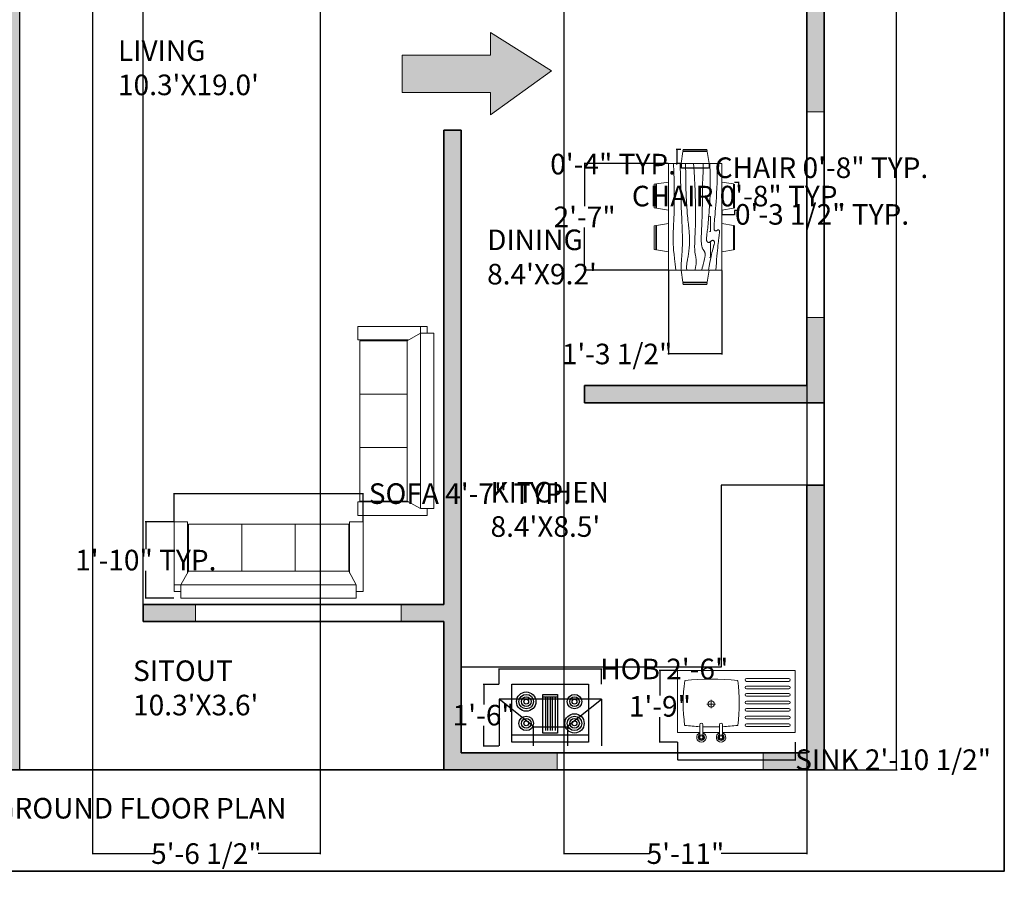
# Model space of a CAD drawing. Units: inches. Extents: x 717 to 1167, y 2046 to 2594.
# Tile 3 of 6: x 880 to 1167, y 2046 to 2298. Entities that reach past the tile are written whole.
import ezdxf

# ---------------------------------------------------------------- set-up
doc = ezdxf.new("R2010")
doc.units = ezdxf.units.IN
doc.header["$MEASUREMENT"] = 0
for name, color, linetype, lineweight in [('A-ANNO-DIMS', 2, 'Continuous', 18), ('A-ANNO-SYMB', 7, 'Continuous', 18), ('A-ANNO-TEXT', 7, 'Continuous', 25), ('A-ANNO-TTLB', 7, 'Continuous', 35), ('A-AREA-IDEN', 7, 'Continuous', 18), ('A-EQPM', 8, 'Continuous', 25), ('A-FLOR-CASE', 8, 'Continuous', 25), ('A-FLOR-FIXT', 8, 'Continuous', 18), ('A-FURN', 8, 'Continuous', 18), ('A-GLAZ', 4, 'Continuous', 18), ('A-WALL', 7, 'Continuous', 35), ('A-WALL-PATT', 140, 'Continuous', 13)]:
    doc.layers.add(name, color=color, linetype=linetype, lineweight=lineweight)
doc.styles.get("Standard").update_dxf_attribs({"font": 'arial.ttf'})
doc.dimstyles.get("Standard").update_dxf_attribs({"dimtxt": 6, "dimasz": 0.18, "dimexe": 0.18, "dimexo": 0.0625, "dimgap": 0.09, "dimtad": 0, "dimtih": 1, "dimtoh": 1, "dimdec": 1, "dimzin": 0, "dimdsep": 46, "dimlunit": 3, "dimtxsty": 'Standard', "dimcen": 0.09, "dimadec": 0, "dimazin": 0, "dimtfac": 1, "dimtdec": 1, "dimtofl": 0, "dimtmove": 0, "dimatfit": 3, "dimfxl": 1, "dimtolj": 1, "dimtzin": 0, "dimarcsym": 0})

# ---------------------------------------------------------------- blocks, each defined once
blk = doc.blocks.new('chimmne')
for p, q in [((17.89, 6.07), (-18.11, 6.07)), ((-18.11, 6.07), (-18.11, -10.43)), ((-6.16, -3.43), (-18.11, 6.07)), ((5.94, -3.43), (17.89, 6.07)), ((17.89, 6.07), (17.89, -10.43)), ((-6.16, -3.43), (-6.16, -10.43)), ((5.94, -3.43), (5.94, -10.43)), ((5.94, -3.82), (-6.16, -3.82))]:
    blk.add_line(p, q)
for points in [[(-13.61, -9.12), (-13.61, 11.28), (13.39, 11.28), (13.39, -9.12)], [(-2.66, -5.87), (-2.66, 7.73), (2.44, 7.73), (2.44, -5.87)]]:
    blk.add_lwpolyline(points, close=True)
for points in [[(-2.66, 6.88), (2.44, 6.88)], [(-1.81, 6.88), (-1.81, -5.02)], [(-0.96, -5.02), (-0.96, 6.88)], [(-0.11, 6.88), (-0.11, -5.02)], [(0.74, -5.02), (0.74, 6.88)], [(1.59, 6.88), (1.59, -5.02)], [(13.39, -6.57), (-13.61, -6.57)]]:
    blk.add_lwpolyline(points)
for centre, radius in [((-8.55, 5.18), 3.4), ((-8.55, 5.18), 2.55), ((8.44, 5.18), 2.55), ((-8.55, 5.18), 1.7), ((-8.55, 5.18), 0.85), ((8.44, 5.18), 1.7), ((8.44, 5.18), 0.85), ((-8.55, -2.47), 2.55), ((8.44, -2.47), 3.4), ((8.44, -2.47), 2.55), ((-8.55, -2.47), 1.7), ((-8.55, -2.47), 0.85), ((8.44, -2.47), 1.7), ((8.44, -2.47), 0.85)]:
    blk.add_circle(centre, radius)
blk = doc.blocks.new('A$C799204C7')
for p, q in [((0, 34.2), (17.99, 34.2)), ((0, 0), (0, 34.2)), ((2.32, 20.01), (2.32, 32.27)), ((3.13, 20.01), (3.13, 32.27)), ((4.48, 20.01), (4.48, 32.27)), ((5.29, 20.01), (5.29, 32.27)), ((6.64, 20.01), (6.64, 32.27)), ((7.45, 20.01), (7.45, 32.27)), ((8.85, 20.01), (8.85, 32.27)), ((9.66, 20.01), (9.66, 32.27)), ((11.01, 20.01), (11.01, 32.27)), ((11.82, 20.01), (11.82, 32.27)), ((13.22, 20.01), (13.22, 32.27)), ((14.03, 20.01), (14.03, 32.27)), ((15.42, 20.01), (15.42, 32.27)), ((16.24, 20.01), (16.24, 32.27)), ((17.99, 13.08), (17.99, 34.2)), ((18.59, 13.08), (15.71, 13.08)), ((15.71, 12.17), (18.59, 12.17)), ((17.99, 7.36), (17.99, 12.17)), ((8.52, 9.77), (10.9, 9.77)), ((9.73, 11), (9.73, 8.54)), ((18.59, 7.36), (15.71, 7.36)), ((15.71, 6.45), (18.59, 6.45)), ((17.99, 0), (17.99, 6.45)), ((0, 0), (17.99, 0))]:
    blk.add_line(p, q)
for centre, radius in [((19.38, 12.62), 0.684), ((19.38, 12.62), 0.456), ((9.7, 9.77), 0.916), ((19.38, 6.91), 0.684), ((19.38, 6.91), 0.456)]:
    blk.add_circle(centre, radius)
for centre, radius, start, end in [((2.72, 32.27), 0.407, 0, 180), ((4.88, 32.27), 0.407, 0, 180), ((7.05, 32.27), 0.407, 0, 180), ((9.25, 32.27), 0.407, 0, 180), ((11.42, 32.27), 0.407, 0, 180), ((13.62, 32.27), 0.407, 0, 180), ((15.83, 32.27), 0.407, 0, 180), ((2.72, 20.01), 0.407, 180, 0), ((67.33, 9.77), 64.88, 173.1952, 186.8048), ((9.53, -30.19), 48.1, 82.3437, 97.8966), ((4.88, 20.01), 0.407, 180, 0), ((7.05, 20.01), 0.407, 180, 0), ((9.25, 20.01), 0.407, 180, 0), ((11.42, 20.01), 0.407, 180, 0), ((13.62, 20.01), 0.407, 180, 0), ((15.83, 20.01), 0.407, 180, 0), ((-48.51, 9.77), 64.88, 2.9208, 6.8048), ((15.71, 12.62), 0.456, 90, 270), ((-48.51, 9.77), 64.88, 357.8723, 2.115), ((19.38, 12.62), 1.37, 199.6514, 160.3603), ((19.38, 12.62), 0.911, 210.3431, 149.7554), ((15.71, 6.91), 0.456, 90, 270), ((-48.51, 9.77), 64.88, 353.1952, 357.0665), ((19.38, 6.91), 1.37, 199.6514, 160.3603), ((19.38, 6.91), 0.911, 210.3431, 149.7554), ((9.53, 49.73), 48.1, 262.1034, 277.6563)]:
    blk.add_arc(centre, radius, start, end)
blk = doc.blocks.new('*D5')
at = {"layer": 'A-ANNO-DIMS', "color": 0, "lineweight": -2, "transparency": 16777216}
for p, q in [((1114.78, 2547.57), (1135.98, 2547.57)), ((1135.8, 2547.39), (1135.8, 2316.73)), ((1135.8, 2079.75), (1135.8, 2310.41)), ((1114.78, 2079.57), (1135.98, 2079.57))]:
    blk.add_line(p, q, dxfattribs=at)
at = {"layer": 'A-ANNO-DIMS', "color": 0, "transparency": 16777216}
for points in [[(1135.77, 2547.39), (1135.83, 2547.39), (1135.8, 2547.57)], [(1135.77, 2079.75), (1135.83, 2079.75), (1135.8, 2079.57)]]:
    blk.add_solid(points, dxfattribs=at)
at = {"layer": 'Defpoints', "color": 0, "transparency": 16777216}
for p in [(1114.71, 2547.57), (1114.71, 2079.57), (1135.8, 2079.57)]:
    blk.add_point(p, dxfattribs=at)
at = {"layer": 'A-ANNO-DIMS', "color": 0, "transparency": 16777216, "insert": (1135.8, 2313.57), "char_height": 6, "attachment_point": 5}
blk.add_mtext("\\A1;39'", dxfattribs=at)
blk = doc.blocks.new('SOFA-3-SEAT')
for p, q in [((0, 1.96), (0, 22.23)), ((3.92, 22.23), (0, 22.23)), ((3.92, 7.54), (3.92, 22.23)), ((4.17, 21.57), (4.17, 7.85)), ((19.74, 21.57), (19.74, 7.85)), ((35.31, 21.57), (35.31, 7.85)), ((51.12, 7.28), (51.12, 22.23)), ((51.12, 22.23), (55.04, 22.23)), ((55.04, 1.96), (55.04, 22.23)), ((1.96, 3.92), (4.17, 7.85)), ((50.88, 7.85), (53.08, 3.92)), ((0, 3.92), (53.08, 3.92)), ((1.96, 3.92), (1.96, 0)), ((53.08, 3.92), (53.08, 0)), ((0, 1.96), (1.96, 1.96)), ((53.08, 1.96), (55.04, 1.96)), ((1.96, 0), (53.08, 0))]:
    blk.add_line(p, q)
blk.add_lwpolyline([(4.17, 7.85), (50.88, 7.85), (50.88, 21.57), (4.17, 21.57)])
blk = doc.blocks.new('CHAIR-DINING')
for p, q in [((0, 7.56), (0.43, 7.63)), ((0, 7.56), (0, 0.64)), ((0.43, 0.57), (0.43, 7.62)), ((0.65, 7.66), (4.11, 8.2)), ((0.65, 7.66), (0.65, 0.54)), ((0.43, 0.57), (0, 0.64)), ((4.11, 0), (0.65, 0.54))]:
    blk.add_line(p, q)
blk = doc.blocks.new('CHAIR-DINING-PARTLY-OCCLUDED')
for p, q in [((3.46, 7.66), (0, 8.2)), ((3.46, 7.66), (3.46, 0.54)), ((3.68, 0.57), (3.68, 7.62)), ((0, 0), (3.46, 0.54))]:
    blk.add_line(p, q)
blk = doc.blocks.new('WINDOW-60IN')
for p, q in [((0, 5), (0, 0)), ((60, 5), (0, 5)), ((60, 0), (60, 5)), ((0, 0), (60, 0))]:
    blk.add_line(p, q)
blk = doc.blocks.new('*D19')
at = {"layer": 'A-ANNO-DIMS', "color": 0, "lineweight": -2, "transparency": 16777216}
for p, q in [((925.32, 2151.89), (925.32, 2160.26)), ((925.5, 2160.08), (980.18, 2160.08)), ((980.36, 2151.89), (980.36, 2160.26)), ((980.36, 2160.08), (980.54, 2160.08))]:
    blk.add_line(p, q, dxfattribs=at)
at = {"layer": 'A-ANNO-DIMS', "color": 0, "transparency": 16777216}
for points in [[(925.5, 2160.11), (925.5, 2160.05), (925.32, 2160.08)], [(980.18, 2160.11), (980.18, 2160.05), (980.36, 2160.08)]]:
    blk.add_solid(points, dxfattribs=at)
at = {"layer": 'Defpoints', "color": 0, "transparency": 16777216}
for p in [(980.36, 2160.08), (925.32, 2151.83), (980.36, 2151.83)]:
    blk.add_point(p, dxfattribs=at)
at = {"layer": 'A-ANNO-DIMS', "color": 0, "transparency": 16777216, "insert": (1011.48, 2160.08), "char_height": 6, "attachment_point": 5}
blk.add_mtext('\\A1;SOFA 4\'-7" TYP.', dxfattribs=at)
blk = doc.blocks.new('*D20')
at = {"layer": 'A-ANNO-DIMS', "color": 0, "lineweight": -2, "transparency": 16777216}
for p, q in [((925.26, 2151.83), (916.88, 2151.83)), ((917.06, 2151.65), (917.06, 2143.86)), ((917.06, 2129.78), (917.06, 2137.56)), ((925.26, 2129.6), (916.88, 2129.6))]:
    blk.add_line(p, q, dxfattribs=at)
at = {"layer": 'A-ANNO-DIMS', "color": 0, "transparency": 16777216}
for points in [[(917.03, 2151.65), (917.09, 2151.65), (917.06, 2151.83)], [(917.03, 2129.78), (917.09, 2129.78), (917.06, 2129.6)]]:
    blk.add_solid(points, dxfattribs=at)
at = {"layer": 'Defpoints', "color": 0, "transparency": 16777216}
for p in [(917.06, 2151.83), (925.32, 2151.83), (925.32, 2129.6)]:
    blk.add_point(p, dxfattribs=at)
at = {"layer": 'A-ANNO-DIMS', "color": 0, "transparency": 16777216, "insert": (917.06, 2140.71), "char_height": 6, "attachment_point": 5}
blk.add_mtext('\\A1;1\'-10" TYP.', dxfattribs=at)
blk = doc.blocks.new('*D23')
at = {"layer": 'A-ANNO-DIMS', "color": 0, "lineweight": -2, "transparency": 16777216}
for p, q in [((1073.01, 2256.23), (1073.01, 2254.88)), ((1073.19, 2255.06), (1081.03, 2255.06)), ((1081.21, 2256.23), (1081.21, 2254.88)), ((1081.21, 2255.06), (1081.39, 2255.06))]:
    blk.add_line(p, q, dxfattribs=at)
at = {"layer": 'A-ANNO-DIMS', "color": 0, "transparency": 16777216}
for points in [[(1073.19, 2255.09), (1073.19, 2255.03), (1073.01, 2255.06)], [(1081.03, 2255.09), (1081.03, 2255.03), (1081.21, 2255.06)]]:
    blk.add_solid(points, dxfattribs=at)
at = {"layer": 'Defpoints', "color": 0, "transparency": 16777216}
for p in [(1073.01, 2256.29), (1081.21, 2256.29), (1081.21, 2255.06)]:
    blk.add_point(p, dxfattribs=at)
at = {"layer": 'A-ANNO-DIMS', "color": 0, "transparency": 16777216, "insert": (1113.94, 2255.06), "char_height": 6, "attachment_point": 5}
blk.add_mtext('\\A1;CHAIR 0\'-8" TYP.', dxfattribs=at)
blk = doc.blocks.new('*D24')
at = {"layer": 'A-ANNO-DIMS', "color": 0, "lineweight": -2, "transparency": 16777216}
for p, q in [((1072.95, 2260.4), (1071.6, 2260.4)), ((1071.78, 2260.22), (1071.78, 2256.47)), ((1072.95, 2256.29), (1071.6, 2256.29)), ((1071.78, 2256.11), (1071.6, 2256.11)), ((1071.78, 2256.29), (1071.78, 2256.11))]:
    blk.add_line(p, q, dxfattribs=at)
at = {"layer": 'A-ANNO-DIMS', "color": 0, "transparency": 16777216}
for points in [[(1071.75, 2260.22), (1071.81, 2260.22), (1071.78, 2260.4)], [(1071.75, 2256.47), (1071.81, 2256.47), (1071.78, 2256.29)]]:
    blk.add_solid(points, dxfattribs=at)
at = {"layer": 'Defpoints', "color": 0, "transparency": 16777216}
for p in [(1073.01, 2260.4), (1071.78, 2256.29), (1073.01, 2256.29)]:
    blk.add_point(p, dxfattribs=at)
at = {"layer": 'A-ANNO-DIMS', "color": 0, "transparency": 16777216, "insert": (1053.22, 2256.11), "char_height": 6, "attachment_point": 5}
blk.add_mtext('\\A1;0\'-4" TYP.', dxfattribs=at)
blk = doc.blocks.new('*D25')
at = {"layer": 'A-ANNO-DIMS', "color": 0, "lineweight": -2, "transparency": 16777216}
for p, q in [((1088.63, 2250.89), (1089.97, 2250.89)), ((1089.79, 2250.71), (1089.79, 2249.98)), ((1089.79, 2242.87), (1089.79, 2243.59)), ((1088.63, 2242.69), (1089.97, 2242.69))]:
    blk.add_line(p, q, dxfattribs=at)
at = {"layer": 'A-ANNO-DIMS', "color": 0, "transparency": 16777216}
for points in [[(1089.76, 2250.71), (1089.82, 2250.71), (1089.79, 2250.89)], [(1089.76, 2242.87), (1089.82, 2242.87), (1089.79, 2242.69)]]:
    blk.add_solid(points, dxfattribs=at)
at = {"layer": 'Defpoints', "color": 0, "transparency": 16777216}
for p in [(1088.57, 2250.89), (1089.79, 2250.89), (1088.57, 2242.69)]:
    blk.add_point(p, dxfattribs=at)
at = {"layer": 'A-ANNO-DIMS', "color": 0, "transparency": 16777216, "insert": (1089.79, 2246.79), "char_height": 6, "attachment_point": 5}
blk.add_mtext('\\A1;CHAIR 0\'-8" TYP.', dxfattribs=at)
blk = doc.blocks.new('*D26')
at = {"layer": 'A-ANNO-DIMS', "color": 0, "lineweight": -2, "transparency": 16777216}
for p, q in [((1084.89, 2242.62), (1084.89, 2241.28)), ((1085.07, 2241.46), (1088.39, 2241.46)), ((1088.57, 2242.62), (1088.57, 2241.28)), ((1088.57, 2241.46), (1088.75, 2241.46))]:
    blk.add_line(p, q, dxfattribs=at)
at = {"layer": 'A-ANNO-DIMS', "color": 0, "transparency": 16777216}
for points in [[(1085.07, 2241.49), (1085.07, 2241.43), (1084.89, 2241.46)], [(1088.39, 2241.49), (1088.39, 2241.43), (1088.57, 2241.46)]]:
    blk.add_solid(points, dxfattribs=at)
at = {"layer": 'Defpoints', "color": 0, "transparency": 16777216}
for p in [(1084.89, 2242.69), (1088.57, 2242.69), (1088.57, 2241.46)]:
    blk.add_point(p, dxfattribs=at)
at = {"layer": 'A-ANNO-DIMS', "color": 0, "transparency": 16777216, "insert": (1114.11, 2241.46), "char_height": 6, "attachment_point": 5}
blk.add_mtext('\\A1;0\'-3 1/2" TYP.', dxfattribs=at)
blk = doc.blocks.new('*D27')
at = {"layer": 'A-ANNO-DIMS', "color": 0, "lineweight": -2, "transparency": 16777216}
for p, q in [((1020, 2104.57), (1020, 2109.16)), ((1020.18, 2108.98), (1049.63, 2108.98)), ((1049.81, 2104.57), (1049.81, 2109.16)), ((1049.81, 2108.98), (1049.99, 2108.98))]:
    blk.add_line(p, q, dxfattribs=at)
at = {"layer": 'A-ANNO-DIMS', "color": 0, "transparency": 16777216}
for points in [[(1020.18, 2109.01), (1020.18, 2108.95), (1020, 2108.98)], [(1049.63, 2109.01), (1049.63, 2108.95), (1049.81, 2108.98)]]:
    blk.add_solid(points, dxfattribs=at)
at = {"layer": 'Defpoints', "color": 0, "transparency": 16777216}
for p in [(1049.81, 2108.98), (1020, 2104.5), (1049.81, 2104.5)]:
    blk.add_point(p, dxfattribs=at)
at = {"layer": 'A-ANNO-DIMS', "color": 0, "transparency": 16777216, "insert": (1068.13, 2108.98), "char_height": 6, "attachment_point": 5}
blk.add_mtext('\\A1;HOB 2\'-6"', dxfattribs=at)
blk = doc.blocks.new('*D28')
at = {"layer": 'A-ANNO-DIMS', "color": 0, "lineweight": -2, "transparency": 16777216}
for p, q in [((1019.93, 2104.5), (1015.34, 2104.5)), ((1015.52, 2104.32), (1015.52, 2098.67)), ((1015.52, 2086.71), (1015.52, 2092.36)), ((1019.93, 2086.53), (1015.34, 2086.53))]:
    blk.add_line(p, q, dxfattribs=at)
at = {"layer": 'A-ANNO-DIMS', "color": 0, "transparency": 16777216}
for points in [[(1015.49, 2104.32), (1015.55, 2104.32), (1015.52, 2104.5)], [(1015.49, 2086.71), (1015.55, 2086.71), (1015.52, 2086.53)]]:
    blk.add_solid(points, dxfattribs=at)
at = {"layer": 'Defpoints', "color": 0, "transparency": 16777216}
for p in [(1015.52, 2104.5), (1020, 2104.5), (1020, 2086.53)]:
    blk.add_point(p, dxfattribs=at)
at = {"layer": 'A-ANNO-DIMS', "color": 0, "transparency": 16777216, "insert": (1015.52, 2095.52), "char_height": 6, "attachment_point": 5}
blk.add_mtext('\\A1;1\'-6"', dxfattribs=at)
blk = doc.blocks.new('*D29')
at = {"layer": 'A-ANNO-DIMS', "color": 0, "lineweight": -2, "transparency": 16777216}
for p, q in [((1072.01, 2087.62), (1072.01, 2082.36)), ((1106.32, 2087.62), (1106.32, 2082.36)), ((1072.19, 2082.54), (1106.14, 2082.54)), ((1106.32, 2082.54), (1106.5, 2082.54))]:
    blk.add_line(p, q, dxfattribs=at)
at = {"layer": 'A-ANNO-DIMS', "color": 0, "transparency": 16777216}
for points in [[(1072.19, 2082.57), (1072.19, 2082.51), (1072.01, 2082.54)], [(1106.14, 2082.57), (1106.14, 2082.51), (1106.32, 2082.54)]]:
    blk.add_solid(points, dxfattribs=at)
at = {"layer": 'Defpoints', "color": 0, "transparency": 16777216}
for p in [(1072.01, 2087.68), (1106.32, 2087.68), (1106.32, 2082.54)]:
    blk.add_point(p, dxfattribs=at)
at = {"layer": 'A-ANNO-DIMS', "color": 0, "transparency": 16777216, "insert": (1134.82, 2082.54), "char_height": 6, "attachment_point": 5}
blk.add_mtext('\\A1;SINK 2\'-10 1/2"', dxfattribs=at)
blk = doc.blocks.new('*D30')
at = {"layer": 'A-ANNO-DIMS', "color": 0, "lineweight": -2, "transparency": 16777216}
for p, q in [((1071.95, 2108.5), (1066.68, 2108.5)), ((1066.86, 2108.32), (1066.86, 2101.25)), ((1066.86, 2087.86), (1066.86, 2094.94)), ((1071.95, 2087.68), (1066.68, 2087.68))]:
    blk.add_line(p, q, dxfattribs=at)
at = {"layer": 'A-ANNO-DIMS', "color": 0, "transparency": 16777216}
for points in [[(1066.83, 2108.32), (1066.89, 2108.32), (1066.86, 2108.5)], [(1066.83, 2087.86), (1066.89, 2087.86), (1066.86, 2087.68)]]:
    blk.add_solid(points, dxfattribs=at)
at = {"layer": 'Defpoints', "color": 0, "transparency": 16777216}
for p in [(1072.01, 2108.5), (1066.86, 2087.68), (1072.01, 2087.68)]:
    blk.add_point(p, dxfattribs=at)
at = {"layer": 'A-ANNO-DIMS', "color": 0, "transparency": 16777216, "insert": (1066.86, 2098.09), "char_height": 6, "attachment_point": 5}
blk.add_mtext('\\A1;1\'-9"', dxfattribs=at)
blk = doc.blocks.new('*D35')
at = {"layer": 'A-ANNO-DIMS', "color": 0, "lineweight": -2, "transparency": 16777216}
for p, q in [((901.51, 2542.51), (901.51, 2054.99)), ((967.91, 2542.51), (967.91, 2054.99)), ((901.69, 2055.17), (919.66, 2055.17)), ((967.73, 2055.17), (949.77, 2055.17))]:
    blk.add_line(p, q, dxfattribs=at)
at = {"layer": 'A-ANNO-DIMS', "color": 0, "transparency": 16777216}
for points in [[(901.69, 2055.2), (901.69, 2055.14), (901.51, 2055.17)], [(967.73, 2055.2), (967.73, 2055.14), (967.91, 2055.17)]]:
    blk.add_solid(points, dxfattribs=at)
at = {"layer": 'Defpoints', "color": 0, "transparency": 16777216}
for p in [(901.51, 2542.57), (967.91, 2542.57), (967.91, 2055.17)]:
    blk.add_point(p, dxfattribs=at)
at = {"layer": 'A-ANNO-DIMS', "color": 0, "transparency": 16777216, "insert": (934.71, 2055.17), "char_height": 6, "attachment_point": 5}
blk.add_mtext('\\A1;5\'-6 1/2"', dxfattribs=at)
blk = doc.blocks.new('*D36')
at = {"layer": 'A-ANNO-DIMS', "color": 0, "lineweight": -2, "transparency": 16777216}
for p, q in [((1038.91, 2357.31), (1038.91, 2054.99)), ((1109.71, 2357.31), (1109.71, 2054.99)), ((1039.09, 2055.17), (1063.92, 2055.17)), ((1109.53, 2055.17), (1084.71, 2055.17))]:
    blk.add_line(p, q, dxfattribs=at)
at = {"layer": 'A-ANNO-DIMS', "color": 0, "transparency": 16777216}
for points in [[(1039.09, 2055.2), (1039.09, 2055.14), (1038.91, 2055.17)], [(1109.53, 2055.2), (1109.53, 2055.14), (1109.71, 2055.17)]]:
    blk.add_solid(points, dxfattribs=at)
at = {"layer": 'Defpoints', "color": 0, "transparency": 16777216}
for p in [(1038.91, 2357.37), (1109.71, 2357.37), (1109.71, 2055.17)]:
    blk.add_point(p, dxfattribs=at)
at = {"layer": 'A-ANNO-DIMS', "color": 0, "transparency": 16777216, "insert": (1074.31, 2055.17), "char_height": 6, "attachment_point": 5}
blk.add_mtext('\\A1;5\'-11"', dxfattribs=at)
blk = doc.blocks.new('*D38')
at = {"layer": 'A-ANNO-DIMS', "color": 0, "lineweight": -2, "transparency": 16777216}
for p, q in [((880.31, 2079.63), (880.31, 2572.15)), ((880.49, 2571.97), (890.25, 2571.97)), ((916.13, 2571.97), (906.38, 2571.97)), ((916.31, 2122.83), (916.31, 2572.15))]:
    blk.add_line(p, q, dxfattribs=at)
at = {"layer": 'A-ANNO-DIMS', "color": 0, "transparency": 16777216}
for points in [[(880.49, 2572), (880.49, 2571.94), (880.31, 2571.97)], [(916.13, 2572), (916.13, 2571.94), (916.31, 2571.97)]]:
    blk.add_solid(points, dxfattribs=at)
at = {"layer": 'Defpoints', "color": 0, "transparency": 16777216}
for p in [(916.31, 2571.97), (916.31, 2122.77), (880.31, 2079.57)]:
    blk.add_point(p, dxfattribs=at)
at = {"layer": 'A-ANNO-DIMS', "color": 0, "transparency": 16777216, "insert": (898.31, 2571.97), "char_height": 6, "attachment_point": 5}
blk.add_mtext('\\A1;3\'-0"', dxfattribs=at)
blk = doc.blocks.new('*D39')
at = {"layer": 'A-ANNO-DIMS', "color": 0, "lineweight": -2, "transparency": 16777216}
for p, q in [((1069.33, 2225.11), (1069.33, 2200.59)), ((1084.89, 2225.11), (1084.89, 2200.59)), ((1069.33, 2200.77), (1069.15, 2200.77)), ((1084.71, 2200.77), (1069.51, 2200.77))]:
    blk.add_line(p, q, dxfattribs=at)
at = {"layer": 'A-ANNO-DIMS', "color": 0, "transparency": 16777216}
for points in [[(1069.51, 2200.8), (1069.51, 2200.74), (1069.33, 2200.77)], [(1084.71, 2200.8), (1084.71, 2200.74), (1084.89, 2200.77)]]:
    blk.add_solid(points, dxfattribs=at)
at = {"layer": 'Defpoints', "color": 0, "transparency": 16777216}
for p in [(1069.33, 2225.17), (1084.89, 2225.17), (1069.33, 2200.77)]:
    blk.add_point(p, dxfattribs=at)
at = {"layer": 'A-ANNO-DIMS', "color": 0, "transparency": 16777216, "insert": (1054.38, 2200.77), "char_height": 6, "attachment_point": 5}
blk.add_mtext('\\A1;1\'-3 1/2"', dxfattribs=at)
blk = doc.blocks.new('*D40')
at = {"layer": 'A-ANNO-DIMS', "color": 0, "lineweight": -2, "transparency": 16777216}
for p, q in [((1069.27, 2256.3), (1044.75, 2256.3)), ((1044.93, 2256.12), (1044.93, 2243.84)), ((1044.93, 2225.35), (1044.93, 2237.63)), ((1069.27, 2225.17), (1044.75, 2225.17))]:
    blk.add_line(p, q, dxfattribs=at)
at = {"layer": 'A-ANNO-DIMS', "color": 0, "transparency": 16777216}
for points in [[(1044.9, 2256.12), (1044.96, 2256.12), (1044.93, 2256.3)], [(1044.9, 2225.35), (1044.96, 2225.35), (1044.93, 2225.17)]]:
    blk.add_solid(points, dxfattribs=at)
at = {"layer": 'Defpoints', "color": 0, "transparency": 16777216}
for p in [(1044.93, 2256.3), (1069.33, 2256.3), (1069.33, 2225.17)]:
    blk.add_point(p, dxfattribs=at)
at = {"layer": 'A-ANNO-DIMS', "color": 0, "transparency": 16777216, "insert": (1044.93, 2240.73), "char_height": 6, "attachment_point": 5}
blk.add_mtext('\\A1;2\'-7"', dxfattribs=at)

msp = doc.modelspace()

# ---------------------------------------------------------------- hatches: boundary and pattern name
at = {"layer": 'A-ANNO-SYMB'}
h = msp.add_hatch(color=256, dxfattribs=at)
h.dxf.hatch_style = 1
h.paths.add_polyline_path([(1035.28, 2283.27), (1017.49, 2294.42), (1017.49, 2287.85), (991.77, 2287.85), (991.77, 2277.02), (1017.49, 2277.02), (1017.49, 2270.45)])
at = {"layer": 'A-WALL-PATT'}
h = msp.add_hatch(color=256, dxfattribs=at)
h.dxf.hatch_style = 1
h.paths.add_polyline_path([(796.2, 2547.57), (754.71, 2547.57), (754.71, 2325.38), (759.71, 2325.38), (759.71, 2357.37), (840.31, 2357.37), (840.31, 2362.37), (759.71, 2362.37), (759.71, 2412.77), (835.31, 2412.77), (835.31, 2386.37), (840.31, 2386.37), (840.31, 2412.77), (901.51, 2412.77), (901.51, 2417.77), (759.71, 2417.77), (759.71, 2542.57), (796.2, 2542.57)])
h.paths.add_polyline_path([(913.34, 2547.57), (856.2, 2547.57), (856.2, 2542.57), (896.51, 2542.57), (896.51, 2453.77), (901.51, 2453.77), (901.51, 2542.57), (913.34, 2542.57)])
h.paths.add_polyline_path([(1012.57, 2547.57), (949.34, 2547.57), (949.34, 2542.57), (967.91, 2542.57), (967.91, 2412.77), (972.91, 2412.77), (972.91, 2542.57), (1012.57, 2542.57)])
h.paths.add_polyline_path([(1114.71, 2547.57), (1072.57, 2547.57), (1072.57, 2542.57), (1109.71, 2542.57), (1109.71, 2517.4), (1114.71, 2517.4)])
h.paths.add_polyline_path([(1114.71, 2457.4), (1109.71, 2457.4), (1109.71, 2393.68), (1114.71, 2393.68)])
h.paths.add_polyline_path([(1114.71, 2369.68), (1109.71, 2369.68), (1109.71, 2362.37), (1038.91, 2362.37), (1038.91, 2412.77), (1085.71, 2412.77), (1085.71, 2417.77), (1008.91, 2417.77), (1008.91, 2412.77), (1033.91, 2412.77), (1033.91, 2362.37), (916.31, 2362.37), (916.31, 2357.37), (1033.91, 2357.37), (1033.91, 2306.97), (1003.91, 2306.97), (1003.91, 2301.97), (1085.71, 2301.97), (1085.71, 2306.97), (1038.91, 2306.97), (1038.91, 2357.37), (1109.71, 2357.37), (1109.71, 2347.44), (1114.71, 2347.44)])
h.paths.add_polyline_path([(788.58, 2239.77), (759.71, 2239.77), (759.71, 2265.38), (754.71, 2265.38), (754.71, 2234.77), (788.58, 2234.77)])
h.paths.add_polyline_path([(880.31, 2362.37), (875.31, 2362.37), (875.31, 2239.77), (848.58, 2239.77), (848.58, 2234.77), (875.31, 2234.77), (875.31, 2079.57), (880.31, 2079.57)])
h.paths.add_polyline_path([(1008.91, 2265.97), (1003.91, 2265.97), (1003.91, 2127.77), (991.51, 2127.77), (991.51, 2122.77), (1003.91, 2122.77), (1003.91, 2079.57), (1036.96, 2079.57), (1036.96, 2084.57), (1008.91, 2084.57)])
h.paths.add_polyline_path([(931.51, 2127.77), (916.31, 2127.77), (916.31, 2122.77), (931.51, 2122.77)])
h.paths.add_polyline_path([(1114.71, 2162.57), (1109.71, 2162.57), (1109.71, 2084.57), (1096.96, 2084.57), (1096.96, 2079.57), (1114.71, 2079.57)])
h.paths.add_polyline_path([(1114.71, 2211.37), (1109.71, 2211.37), (1109.71, 2191.57), (1044.91, 2191.57), (1044.91, 2186.57), (1114.71, 2186.57)])
h.paths.add_polyline_path([(1114.71, 2323.44), (1109.71, 2323.44), (1109.71, 2271.37), (1114.71, 2271.37)])

# ---------------------------------------------------------------- linework, layer by layer
at = {"layer": 'A-ANNO-SYMB'}
for p, q in [((1017.49, 2287.85), (1017.49, 2294.42)), ((1017.49, 2294.42), (1035.28, 2283.27)), ((991.77, 2287.85), (991.77, 2277.02)), ((991.77, 2287.85), (1017.49, 2287.85)), ((1035.28, 2283.27), (1017.49, 2270.45)), ((991.77, 2277.02), (1017.49, 2277.02)), ((1017.49, 2277.02), (1017.49, 2270.45))]:
    msp.add_line(p, q, dxfattribs=at)
at = {"layer": 'A-ANNO-TTLB'}
msp.add_lwpolyline([(719.86, 2594.22), (1167.21, 2594.22), (1167.21, 2050.08), (719.86, 2050.08)], close=True, dxfattribs=at)
at = {"layer": 'A-FLOR-CASE'}
for p, q in [((1109.71, 2162.57), (1084.67, 2162.57)), ((1084.67, 2162.57), (1084.67, 2109.48)), ((1084.67, 2109.48), (1008.91, 2109.48))]:
    msp.add_line(p, q, dxfattribs=at)
at = {"layer": 'A-FURN'}
for p, q in [((1069.33, 2256.3), (1069.33, 2225.17)), ((1084.89, 2256.3), (1069.33, 2256.3)), ((1084.89, 2225.17), (1084.89, 2256.3)), ((1081.59, 2240.8), (1081.32, 2240.84)), ((1081.59, 2240.8), (1081.59, 2236.49)), ((1081.32, 2236.45), (1081.59, 2236.49)), ((1081.59, 2233.26), (1081.32, 2233.3)), ((1081.59, 2233.26), (1081.59, 2228.95)), ((1081.32, 2228.9), (1081.59, 2228.95)), ((1069.33, 2225.17), (1084.89, 2225.17))]:
    msp.add_line(p, q, dxfattribs=at)
for points in [[(1070.84, 2256.3), (1070.91, 2253.74), (1070.97, 2251.55), (1071, 2249.7), (1071.03, 2248.12), (1071.04, 2246.77), (1071.04, 2245.62), (1071.03, 2244.61), (1071.02, 2243.71), (1071.01, 2242.86), (1070.99, 2242.07), (1070.97, 2241.33), (1070.95, 2240.63), (1070.92, 2239.97), (1070.9, 2239.35), (1070.87, 2238.77), (1070.84, 2238.21), (1070.82, 2237.68), (1070.79, 2237.17), (1070.77, 2236.67), (1070.75, 2236.18), (1070.73, 2235.67), (1070.72, 2235.15), (1070.71, 2234.6), (1070.72, 2234.02), (1070.73, 2233.39), (1070.75, 2232.69), (1070.8, 2231.88), (1070.87, 2230.94), (1070.97, 2229.83), (1071.1, 2228.52), (1071.27, 2226.98), (1071.49, 2225.17)], [(1072.79, 2256.3), (1072.87, 2252.15), (1072.95, 2248.72), (1073.03, 2245.91), (1073.1, 2243.65), (1073.17, 2241.82), (1073.23, 2240.35), (1073.28, 2239.14), (1073.33, 2238.1), (1073.36, 2237.16), (1073.39, 2236.28), (1073.41, 2235.47), (1073.42, 2234.73), (1073.42, 2234.04), (1073.42, 2233.4), (1073.41, 2232.82), (1073.4, 2232.27), (1073.38, 2231.76), (1073.37, 2231.28), (1073.35, 2230.83), (1073.32, 2230.39), (1073.29, 2229.97), (1073.27, 2229.55), (1073.23, 2229.13), (1073.2, 2228.7), (1073.17, 2228.26), (1073.13, 2227.82), (1073.1, 2227.36), (1073.07, 2226.91), (1073.04, 2226.46), (1073.02, 2226.02), (1073.01, 2225.59), (1073, 2225.17)], [(1074.3, 2256.3), (1074.38, 2252.48), (1074.46, 2249.42), (1074.54, 2246.99), (1074.62, 2245.1), (1074.7, 2243.66), (1074.77, 2242.57), (1074.84, 2241.71), (1074.91, 2241), (1074.98, 2240.36), (1075.04, 2239.75), (1075.1, 2239.18), (1075.16, 2238.65), (1075.21, 2238.14), (1075.26, 2237.65), (1075.3, 2237.19), (1075.35, 2236.74), (1075.38, 2236.29), (1075.42, 2235.86), (1075.45, 2235.43), (1075.47, 2235.01), (1075.49, 2234.58), (1075.5, 2234.15), (1075.5, 2233.72), (1075.49, 2233.28), (1075.47, 2232.83), (1075.44, 2232.37), (1075.41, 2231.92), (1075.37, 2231.46), (1075.32, 2231.02), (1075.27, 2230.59), (1075.22, 2230.17), (1075.17, 2229.78), (1075.11, 2229.42), (1075.06, 2229.08), (1075, 2228.75), (1074.95, 2228.45), (1074.9, 2228.16), (1074.85, 2227.87), (1074.8, 2227.59), (1074.75, 2227.32), (1074.71, 2227.04), (1074.66, 2226.76), (1074.63, 2226.48), (1074.61, 2226.21), (1074.61, 2225.94), (1074.63, 2225.68), (1074.67, 2225.42), (1074.73, 2225.17)], [(1076.68, 2256.3), (1076.83, 2254.04), (1076.95, 2251.98), (1077.04, 2250.09), (1077.11, 2248.37), (1077.17, 2246.79), (1077.2, 2245.34), (1077.22, 2244.01), (1077.24, 2242.79), (1077.24, 2241.66), (1077.23, 2240.61), (1077.22, 2239.64), (1077.21, 2238.74), (1077.19, 2237.9), (1077.16, 2237.12), (1077.14, 2236.38), (1077.11, 2235.69), (1077.08, 2235.03), (1077.06, 2234.41), (1077.03, 2233.82), (1077.02, 2233.26), (1077, 2232.74), (1076.99, 2232.26), (1076.99, 2231.81), (1077, 2231.4), (1077.02, 2231.03), (1077.05, 2230.69), (1077.08, 2230.38), (1077.12, 2230.09), (1077.16, 2229.83), (1077.2, 2229.59), (1077.25, 2229.36), (1077.29, 2229.14), (1077.33, 2228.92), (1077.36, 2228.71), (1077.39, 2228.51), (1077.42, 2228.3), (1077.43, 2228.09), (1077.44, 2227.87), (1077.44, 2227.64), (1077.43, 2227.41), (1077.42, 2227.16), (1077.39, 2226.9), (1077.36, 2226.65), (1077.32, 2226.4), (1077.28, 2226.17), (1077.25, 2225.95), (1077.21, 2225.77), (1077.18, 2225.62), (1077.16, 2225.51), (1077.14, 2225.44), (1077.13, 2225.39), (1077.12, 2225.35), (1077.11, 2225.32), (1077.11, 2225.29), (1077.11, 2225.24), (1077.11, 2225.17)], [(1079.49, 2256.3), (1079.42, 2254.01), (1079.36, 2252), (1079.32, 2250.24), (1079.29, 2248.7), (1079.27, 2247.35), (1079.26, 2246.16), (1079.25, 2245.1), (1079.24, 2244.16), (1079.22, 2243.29), (1079.2, 2242.49), (1079.18, 2241.75), (1079.16, 2241.05), (1079.13, 2240.4), (1079.11, 2239.77), (1079.08, 2239.17), (1079.06, 2238.57), (1079.03, 2237.98), (1079, 2237.39), (1078.98, 2236.81), (1078.96, 2236.25), (1078.94, 2235.71), (1078.92, 2235.19), (1078.91, 2234.7), (1078.91, 2234.25), (1078.91, 2233.84), (1078.92, 2233.46), (1078.94, 2233.13), (1078.97, 2232.82), (1079, 2232.55), (1079.03, 2232.31), (1079.08, 2232.1), (1079.13, 2231.91), (1079.18, 2231.74), (1079.25, 2231.6), (1079.31, 2231.47), (1079.38, 2231.36), (1079.46, 2231.26), (1079.53, 2231.16), (1079.6, 2231.07), (1079.67, 2230.97), (1079.73, 2230.88), (1079.79, 2230.77), (1079.85, 2230.67), (1079.9, 2230.55), (1079.95, 2230.43), (1079.98, 2230.3), (1080.01, 2230.16), (1080.03, 2230), (1080.04, 2229.83), (1080.04, 2229.65), (1080.02, 2229.46), (1080.01, 2229.26), (1079.98, 2229.05), (1079.94, 2228.83), (1079.9, 2228.61), (1079.85, 2228.38), (1079.79, 2228.14), (1079.72, 2227.89), (1079.65, 2227.61), (1079.56, 2227.28), (1079.46, 2226.88), (1079.34, 2226.41), (1079.21, 2225.84), (1079.06, 2225.17)], [(1081.43, 2256.3), (1081.49, 2253.26), (1081.52, 2250.75), (1081.52, 2248.7), (1081.49, 2247.03), (1081.45, 2245.68), (1081.39, 2244.57), (1081.32, 2243.64), (1081.25, 2242.81), (1081.19, 2242.02), (1081.12, 2241.26), (1081.06, 2240.54), (1081.01, 2239.86), (1080.95, 2239.21), (1080.89, 2238.6), (1080.84, 2238.03), (1080.78, 2237.49), (1080.73, 2237), (1080.68, 2236.54), (1080.63, 2236.13), (1080.58, 2235.75), (1080.54, 2235.41), (1080.51, 2235.1), (1080.48, 2234.82), (1080.46, 2234.57), (1080.45, 2234.36), (1080.45, 2234.17), (1080.46, 2234.01), (1080.48, 2233.87), (1080.51, 2233.75), (1080.55, 2233.65), (1080.59, 2233.57), (1080.64, 2233.49), (1080.7, 2233.43), (1080.76, 2233.38), (1080.83, 2233.34), (1080.9, 2233.31), (1080.98, 2233.29), (1081.06, 2233.29), (1081.14, 2233.29), (1081.22, 2233.31), (1081.3, 2233.35), (1081.38, 2233.39), (1081.46, 2233.44), (1081.54, 2233.5), (1081.62, 2233.56), (1081.7, 2233.63), (1081.78, 2233.69), (1081.87, 2233.75), (1081.95, 2233.8), (1082.03, 2233.84), (1082.11, 2233.87), (1082.18, 2233.89), (1082.26, 2233.91), (1082.34, 2233.9), (1082.41, 2233.89), (1082.48, 2233.85), (1082.54, 2233.81), (1082.6, 2233.74), (1082.66, 2233.66), (1082.7, 2233.57), (1082.74, 2233.47), (1082.76, 2233.35), (1082.77, 2233.23), (1082.77, 2233.1), (1082.74, 2232.96), (1082.71, 2232.81), (1082.66, 2232.63), (1082.59, 2232.44), (1082.52, 2232.21), (1082.43, 2231.95), (1082.34, 2231.64), (1082.24, 2231.28), (1082.14, 2230.86), (1082.03, 2230.38), (1081.9, 2229.81), (1081.76, 2229.14), (1081.61, 2228.35), (1081.43, 2227.44), (1081.23, 2226.39), (1081, 2225.17)], [(1083.59, 2256.3), (1083.58, 2254.21), (1083.56, 2252.32), (1083.51, 2250.61), (1083.46, 2249.07), (1083.39, 2247.67), (1083.32, 2246.39), (1083.24, 2245.24), (1083.16, 2244.17), (1083.08, 2243.19), (1083, 2242.29), (1082.93, 2241.47), (1082.86, 2240.72), (1082.79, 2240.04), (1082.74, 2239.45), (1082.69, 2238.92), (1082.66, 2238.46), (1082.64, 2238.08), (1082.63, 2237.76), (1082.63, 2237.5), (1082.65, 2237.29), (1082.67, 2237.12), (1082.71, 2236.99), (1082.75, 2236.88), (1082.8, 2236.81), (1082.86, 2236.75), (1082.92, 2236.7), (1082.99, 2236.68), (1083.06, 2236.66), (1083.13, 2236.65), (1083.2, 2236.66), (1083.27, 2236.68), (1083.34, 2236.7), (1083.41, 2236.73), (1083.47, 2236.76), (1083.53, 2236.8), (1083.59, 2236.84), (1083.65, 2236.88), (1083.7, 2236.91), (1083.76, 2236.93), (1083.81, 2236.95), (1083.86, 2236.96), (1083.92, 2236.96), (1083.97, 2236.95), (1084.02, 2236.92), (1084.06, 2236.89), (1084.1, 2236.85), (1084.14, 2236.8), (1084.17, 2236.74), (1084.19, 2236.66), (1084.21, 2236.58), (1084.22, 2236.48), (1084.22, 2236.36), (1084.22, 2236.22), (1084.21, 2236.06), (1084.19, 2235.87), (1084.17, 2235.66), (1084.14, 2235.41), (1084.1, 2235.13), (1084.06, 2234.81), (1084.01, 2234.44), (1083.96, 2234.02), (1083.9, 2233.54), (1083.84, 2233), (1083.77, 2232.4), (1083.71, 2231.72), (1083.63, 2230.97), (1083.56, 2230.16), (1083.48, 2229.28), (1083.4, 2228.34), (1083.32, 2227.34), (1083.24, 2226.28), (1083.16, 2225.17)]]:
    msp.add_lwpolyline(points, dxfattribs=at)
at = {"layer": 'A-WALL'}
for p, q in [((1114.71, 2547.57), (1114.71, 2079.57)), ((1109.71, 2357.37), (1109.71, 2191.57)), ((1003.91, 2265.97), (1008.91, 2265.97)), ((1003.91, 2265.97), (1003.91, 2127.77)), ((1008.91, 2265.97), (1008.91, 2084.57)), ((1044.91, 2191.57), (1044.91, 2186.57)), ((1044.91, 2191.57), (1109.71, 2191.57)), ((1044.91, 2186.57), (1114.71, 2186.57)), ((1109.71, 2162.57), (1114.71, 2162.57)), ((1109.71, 2162.57), (1109.71, 2084.57)), ((916.31, 2127.77), (916.31, 2122.77)), ((916.31, 2127.77), (1003.91, 2127.77)), ((916.31, 2122.77), (1003.91, 2122.77)), ((1003.91, 2122.77), (1003.91, 2079.57)), ((1008.91, 2084.57), (1109.71, 2084.57)), ((754.71, 2079.57), (1114.71, 2079.57))]:
    msp.add_line(p, q, dxfattribs=at)

# ---------------------------------------------------------------- block references
at = {"layer": 'A-EQPM', "xscale": 0.8280321260258986, "yscale": 0.8280321260258986, "zscale": 0.8280321260258986}
msp.add_blockref('chimmne', (1034.99, 2095.17), dxfattribs=at)
at = {"layer": 'A-FLOR-FIXT', "xscale": 1.0032, "yscale": 1.0032, "zscale": 1.0032, "rotation": 270}
msp.add_blockref('A$C799204C7', (1072.01, 2108.5), dxfattribs=at)
at = {"layer": 'A-FURN'}
for p, rotation in [((1073.01, 2260.4), 270.0000441632001), ((1081.21, 2221.07), 89.99413959734746)]:
    msp.add_blockref('CHAIR-DINING', p, dxfattribs=dict(at, rotation=rotation))
for name, p in [('CHAIR-DINING', (1065.22, 2242.69)), ('CHAIR-DINING-PARTLY-OCCLUDED', (1084.89, 2242.69)), ('CHAIR-DINING', (1065.22, 2230.58)), ('CHAIR-DINING-PARTLY-OCCLUDED', (1084.89, 2230.58)), ('SOFA-3-SEAT', (925.32, 2129.6))]:
    msp.add_blockref(name, p, dxfattribs=at)
at = {"layer": 'A-FURN', "extrusion": (0, 0, -1), "zscale": -1, "rotation": 270.0000000000025}
msp.add_blockref('SOFA-3-SEAT', (-1001.03, 2208.79), dxfattribs=at)
at = {"layer": 'A-GLAZ', "rotation": 270}
msp.add_blockref('WINDOW-60IN', (1109.71, 2271.37), dxfattribs=at)
at = {"layer": 'A-GLAZ'}
for p in [(931.51, 2122.77), (1036.96, 2079.57)]:
    msp.add_blockref('WINDOW-60IN', p, dxfattribs=at)

# ---------------------------------------------------------------- texts
at = {"layer": 'A-ANNO-TEXT', "insert": (873.16, 2071.4), "char_height": 6, "attachment_point": 1}
msp.add_mtext_dynamic_manual_height_columns('GROUND FLOOR PLAN', width=108.3217, gutter_width=30, heights=[0], dxfattribs=at)
at = {"layer": 'A-AREA-IDEN', "char_height": 6, "attachment_point": 1}
for s, width, insert in [("LIVING\\P10.3'X19.0'", 64.6446, (908.96, 2292.2)), ("DINING\\P8.4'X9.2'", 42.1615, (1016.51, 2237.04)), ("KITCHEN\\P8.4'X8.5'", 52.2808, (1017.51, 2163.49)), ("SITOUT\\P10.3'X3.6'", 47.7379, (913.35, 2111.46))]:
    msp.add_mtext_dynamic_manual_height_columns(s, width=width, gutter_width=30, heights=[0], dxfattribs=dict(at, insert=insert))

# ---------------------------------------------------------------- dimensions: what is measured, and where the dimension line sits
at = {"layer": 'A-ANNO-DIMS'}
for base, p1, p2, picture, middle in [((916.31, 2571.97), (880.31, 2079.57), (916.31, 2122.77), '*D38', (898.31, 2571.97)), ((967.91, 2055.17), (901.51, 2542.57), (967.91, 2542.57), '*D35', (934.71, 2055.17)), ((1109.71, 2055.17), (1038.91, 2357.37), (1109.71, 2357.37), '*D36', (1074.31, 2055.17))]:
    dim = msp.add_linear_dim(base=base, p1=p1, p2=p2, dimstyle='Standard', override={"dimdec": 1, "dimlfac": 1, "dimrnd": 0, "dimzin": 1, "dimdsep": 46, "dimlunit": 4, "dimfrac": 2}, dxfattribs=at)
    dim.commit()
    dim.dimension.update_dxf_attribs({"geometry": picture, "text_midpoint": middle})
for base, p1, p2, angle, override, picture, middle in [((1135.8, 2079.57), (1114.71, 2547.57), (1114.71, 2079.57), 90, {"dimclrd": 0, "dimclre": 0, "dimclrt": 0}, '*D5', (1135.8, 2313.57)), ((1044.93, 2256.3), (1069.33, 2225.17), (1069.33, 2256.3), 90, {"dimdec": 1, "dimlfac": 1, "dimrnd": 0, "dimzin": 1, "dimdsep": 46, "dimlunit": 4, "dimfrac": 2}, '*D40', (1044.93, 2240.73)), ((1069.33, 2200.77), (1084.89, 2225.17), (1069.33, 2225.17), 180, {"dimdec": 1, "dimlfac": 1, "dimrnd": 0, "dimzin": 1, "dimdsep": 46, "dimlunit": 4, "dimfrac": 2}, '*D39', (1054.38, 2200.77)), ((1066.86, 2087.68), (1072.01, 2108.5), (1072.01, 2087.68), 270, {"dimdec": 1, "dimlfac": 1, "dimrnd": 0, "dimzin": 1, "dimdsep": 46, "dimlunit": 4, "dimfrac": 2}, '*D30', (1066.86, 2098.09)), ((1015.52, 2104.5), (1020, 2086.53), (1020, 2104.5), 90, {"dimdec": 1, "dimlfac": 1, "dimrnd": 0, "dimzin": 1, "dimdsep": 46, "dimlunit": 4, "dimfrac": 2}, '*D28', (1015.52, 2095.52))]:
    dim = msp.add_linear_dim(base=base, p1=p1, p2=p2, angle=angle, dimstyle='Standard', override=override, dxfattribs=at)
    dim.commit()
    dim.dimension.update_dxf_attribs({"geometry": picture, "text_midpoint": middle})
for base, p1, p2, angle, text, picture, middle in [((1081.21, 2255.06), (1073.01, 2256.29), (1081.21, 2256.29), 0, 'CHAIR <> TYP.', '*D23', (1113.94, 2255.06)), ((1071.78, 2256.29), (1073.01, 2260.4), (1073.01, 2256.29), 270, '<> TYP.', '*D24', (1053.22, 2256.11)), ((1089.79, 2250.89), (1088.57, 2242.69), (1088.57, 2250.89), 90, 'CHAIR <> TYP.', '*D25', (1089.79, 2246.79)), ((917.06, 2151.83), (925.32, 2129.6), (925.32, 2151.83), 90, '<> TYP.', '*D20', (917.06, 2140.71))]:
    dim = msp.add_linear_dim(base=base, p1=p1, p2=p2, angle=angle, text=text, dimstyle='Standard', override={"dimdec": 1, "dimlfac": 1, "dimrnd": 0, "dimzin": 1, "dimdsep": 46, "dimlunit": 4, "dimfrac": 2}, dxfattribs=at)
    dim.commit()
    dim.dimension.update_dxf_attribs({"geometry": picture, "text_midpoint": middle})
for base, p1, p2, text, picture, middle in [((1088.57, 2241.46), (1084.89, 2242.69), (1088.57, 2242.69), '<> TYP.', '*D26', (1114.11, 2241.46)), ((980.36, 2160.08), (925.32, 2151.83), (980.36, 2151.83), 'SOFA <> TYP.', '*D19', (1011.48, 2160.08)), ((1049.81, 2108.98), (1020, 2104.5), (1049.81, 2104.5), 'HOB <>', '*D27', (1068.13, 2108.98)), ((1106.32, 2082.54), (1072.01, 2087.68), (1106.32, 2087.68), 'SINK <>', '*D29', (1134.82, 2082.54))]:
    dim = msp.add_linear_dim(base=base, p1=p1, p2=p2, text=text, dimstyle='Standard', override={"dimdec": 1, "dimlfac": 1, "dimrnd": 0, "dimzin": 1, "dimdsep": 46, "dimlunit": 4, "dimfrac": 2}, dxfattribs=at)
    dim.commit()
    dim.dimension.update_dxf_attribs({"geometry": picture, "text_midpoint": middle})

doc.saveas('drawing.dxf')
